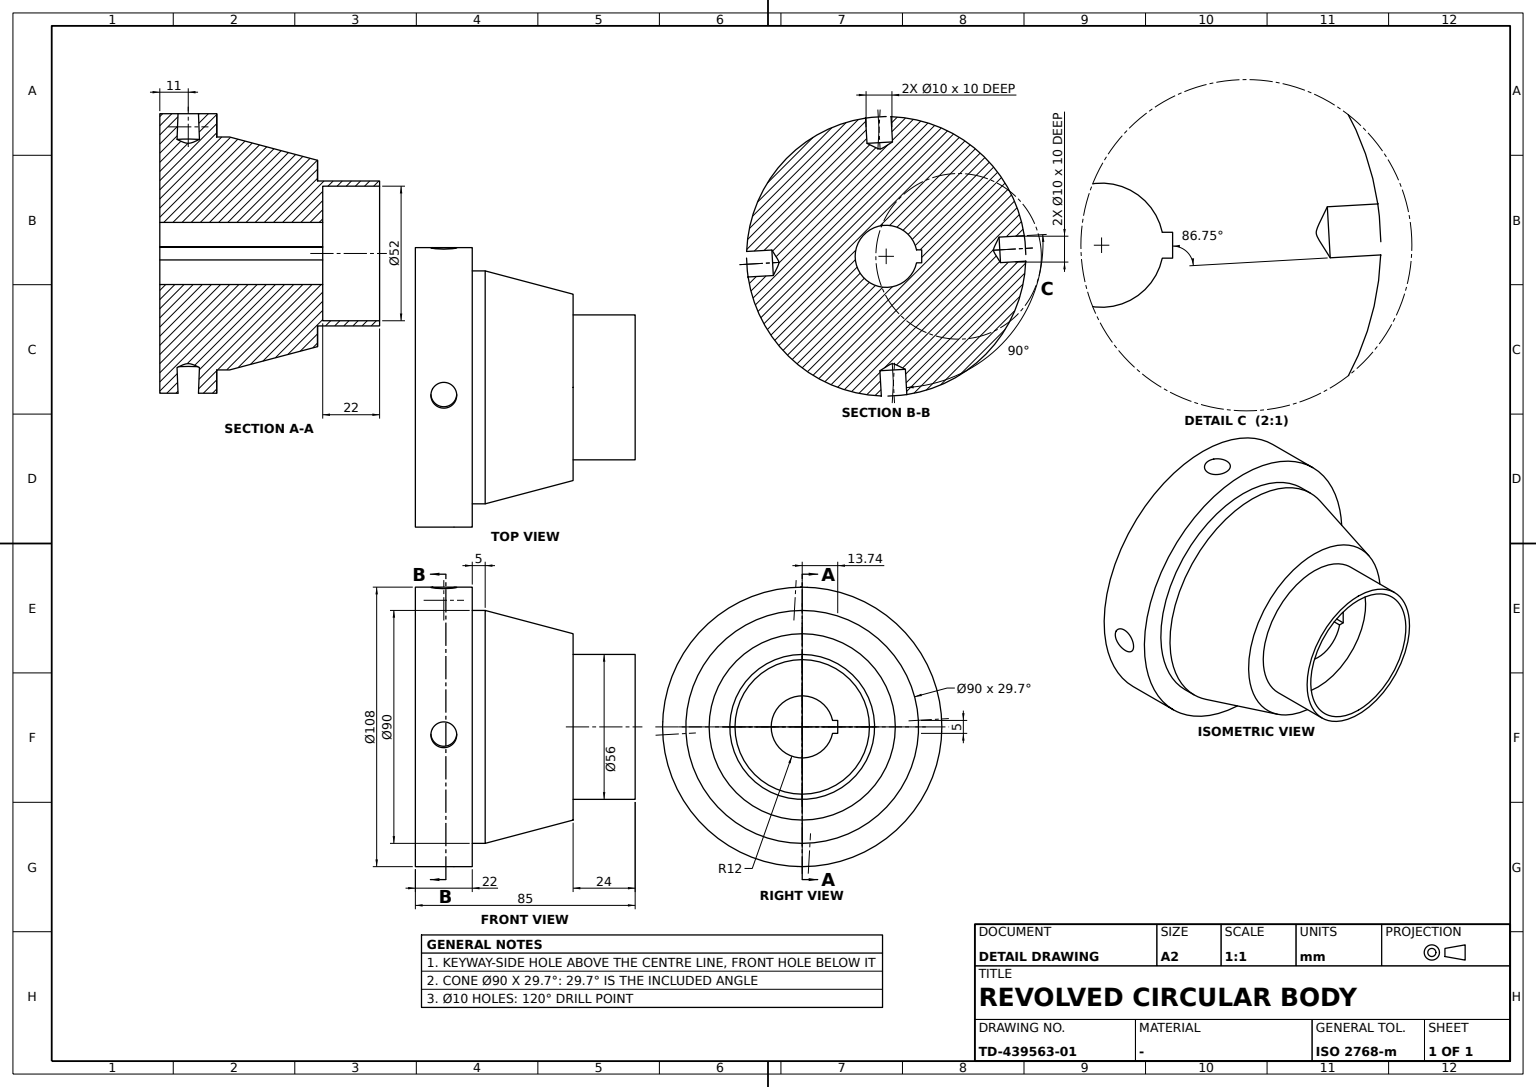
CATIA V5 part; units mm, degrees
sketch "Sketch1" plane through (0, 0, 0) normal (0, 1, 0) x (-1, 0, 0)
  line L0 (0, 0) -> (0, 28)
  line L1 (0, 28) -> (24, 28)
  line L2 (24, 28) -> (24, 36)
  point P0 (24, 36)
  point P1 (24, 36)
  line L3 (24, 36) -> (58, 45)
  line L4 (58, 45) -> (63, 45)
  line L5 (63, 45) -> (63, 54)
  line L6 (63, 54) -> (85, 54)
  line L7 (85, 54) -> (85, 0)
  point P2 (85, 0)
  line L8 (85, 0) -> (0, 0)
  dimension "length L0" = 28
  dimension "length L1" = 24
  dimension "length L6" = 22
  dimension "distance P0 L8" = 36
  dimension "distance L6 L8" = 54
  dimension "distance L4 L8" = 45
  dimension "length L4" = 5
  dimension "distance L0 L7" = 85
  constraint vertical L0 y-axis
  constraint vertical L2 y-axis
  constraint vertical L5 y-axis
  constraint vertical L7 y-axis
  constraint horizontal L1 x-axis
  constraint horizontal L4 x-axis
  constraint horizontal L6 x-axis
  constraint horizontal L8 x-axis
  constraint coincidence P2 x-axis
  constraint coincidence P0 P1
revolve "Shaft1" add sketch "Sketch1" angle 360 about L8
sketch "Sketch2" plane through (0, 0, 0) normal (1, 0, 0) x (0, 1, 0)
  circle A0 centre (0, 0) radius 26
  point P0 (0, -26)
  dimension "radius A0" = 26
  constraint coincidence A0 P0
  constraint coincidence P0 y-axis
extrude "Pocket1" cut sketch "Sketch2" against normal blind 22
sketch "Sketch3" plane through (-22, 0, 0) normal (1, 0, 0) x (0, 1, 0)
  arc A0 (11.7367, 2.5) -> (11.7367, -2.5) centre (0, 0) ccw
  line L0 (11.7367, 2.5) -> (13.7367, 2.5)
  line L1 (13.7367, 2.5) -> (13.7367, -2.5)
  line L2 (13.7367, -2.5) -> (11.7367, -2.5)
  dimension "radius A0" = 12
  dimension "length L0" = 2
  dimension "length L1" = 5
  constraint horizontal L0 x-axis
  constraint horizontal L2 x-axis
  constraint vertical L1 y-axis
  constraint symmetry L0 L2 x-axis
extrude "Pocket2" cut sketch "Sketch3" against normal through all
sketch "Sketch4" plane through (-73.2994, 53.9131, 3.0626) normal (0, -0.9984, -0.0567) x (1, 0, 0)
  point P0 (-0.7006, 0)
  line L0 (-11.7006, -54) -> (-11.7006, 54) construction
  dimension "distance P0 L0" = 11
  dimension "D2" = 0
hole "Hole1" at (-74, 53.9131, 3.0626) direction (0, -0.9984, -0.0567) diameter 10 depth 10 tip angle 120
pattern_circular "CircPattern1" count 4 over 360 about axis through (-85, 0, 0) along (1, 0, 0) of "Hole1"
equation "\"angular step@CircPattern1\" = 360.0*1 deg/CircPattern1.AngularNumber"
